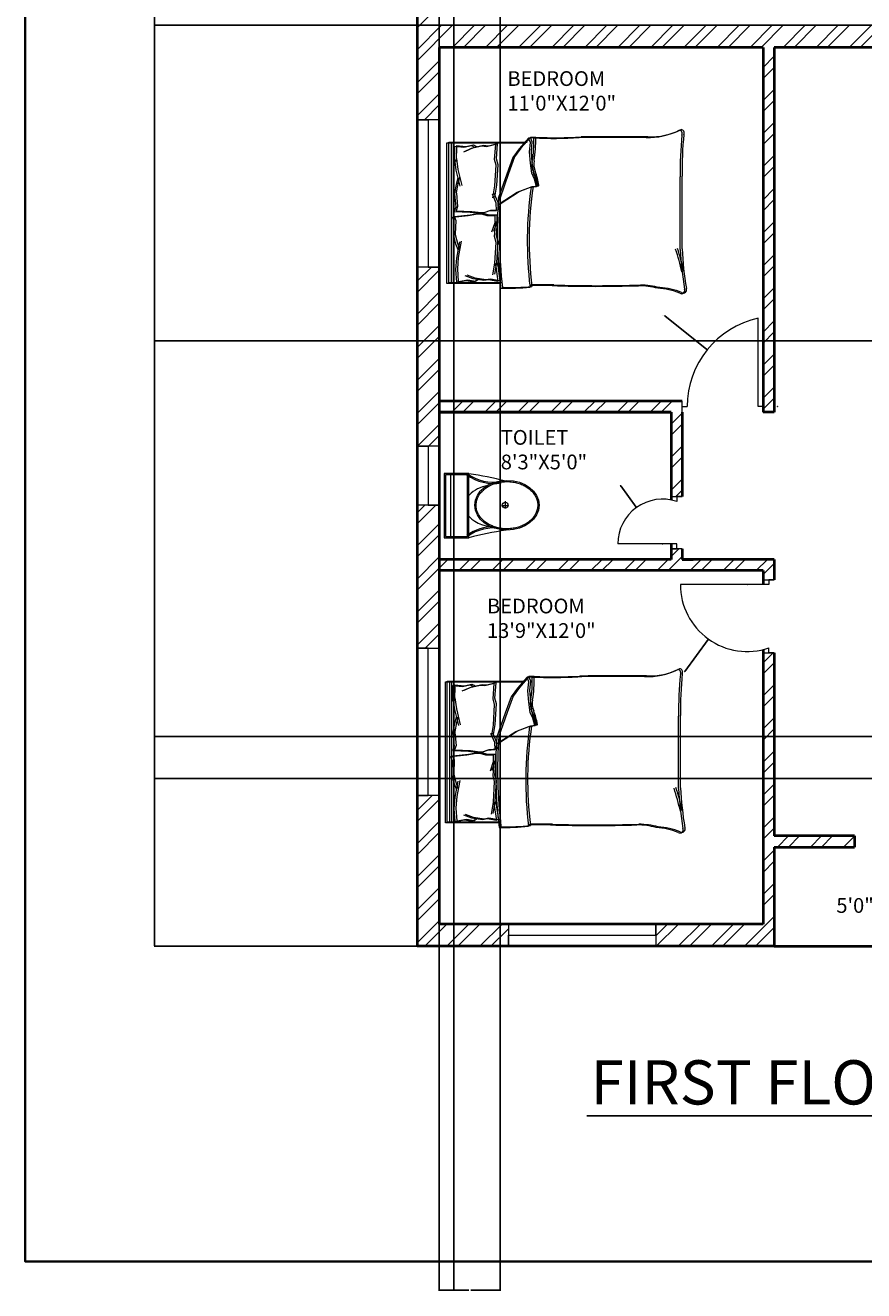
# Model space of a CAD drawing. Units: inches. Extents: x 1355 to 2746, y 1171 to 2751.
# Tile 1 of 24: x 1355 to 1697, y 1171 to 1686. Entities that reach past the tile are written whole.
import ezdxf

# ---------------------------------------------------------------- set-up
doc = ezdxf.new("R2010")
doc.units = ezdxf.units.IN
for name, color, linetype, lineweight in [('A-ANNO-DIMS', 2, 'Continuous', 18), ('A-ANNO-TITL', 7, 'Continuous', 25), ('A-ANNO-TTLB', 7, 'Continuous', 35), ('A-AREA-IDEN', 7, 'Continuous', 18), ('A-DOOR', 3, 'Continuous', 20), ('A-FLOR-FIXT', 9, 'Continuous', 18), ('A-FURN', 8, 'Continuous', 13), ('A-GLAZ', 4, 'Continuous', 18), ('A-WALL', 7, 'Continuous', 40), ('A-WALL-PATT', 252, 'Continuous', 13)]:
    doc.layers.add(name, color=color, linetype=linetype, lineweight=lineweight)
doc.styles.get("Standard").update_dxf_attribs({"font": 'arial.ttf'})
doc.dimstyles.get("Standard").update_dxf_attribs({"dimtxt": 0.18, "dimasz": 0.18, "dimexe": 0.18, "dimexo": 0.0625, "dimgap": 0.09, "dimtad": 0, "dimtih": 1, "dimtoh": 1, "dimdec": 4, "dimzin": 0, "dimdsep": 46, "dimtxsty": 'Standard', "dimcen": 0.09, "dimadec": 0, "dimazin": 0, "dimtfac": 1, "dimtdec": 4, "dimtofl": 0, "dimtmove": 0, "dimatfit": 3, "dimfxl": 1, "dimtolj": 1, "dimtzin": 0, "dimarcsym": 0})

# ---------------------------------------------------------------- blocks, each defined once
blk = doc.blocks.new('A$C31115884')
for p, q in [((258, 466), (258, 523)), ((283, 498), (223, 498)), ((0, 200), (0, 0)), ((520, 200), (0, 200)), ((10, 190), (10, 10)), ((510, 190), (10, 190)), ((510, 10), (510, 190)), ((520, 0), (520, 200)), ((510, 54), (0, 54)), ((10, 10), (510, 10)), ((0, 0), (520, 0))]:
    blk.add_line(p, q)
blk.add_circle((256, 496), 23.6)
for centre, radius, start, end in [((2778, -205), 2807, 165.4549, 171.7133), ((-295, 403), 365, 324.2091, 9.3499), ((-295, 403), 375, 324.2091, 9.3499), ((139, 406), 293, 315.8436, 2.6563), ((806, 403), 365, 170.6501, 215.7909), ((3237, 905), 2807, 188.2867, 194.5451), ((384, 406), 293, 190.2774, 224.1564), ((806, 403), 375, 179.2036, 215.7909)]:
    blk.add_arc(centre, radius, start, end)
blk.add_ellipse((256, 510), major_axis=(0, -261), ratio=0.772727)
blk.add_open_spline([(256, 259), (263, 259), (270, 260), (288, 262), (299, 265), (320, 273), (330, 278), (350, 291), (360, 299), (378, 316), (386, 326), (402, 347), (409, 358), (421, 383), (427, 395), (436, 422), (440, 436), (445, 465), (447, 480), (448, 509), (448, 524), (445, 553), (443, 568), (436, 596), (432, 610), (422, 636), (416, 649), (402, 672), (395, 683), (379, 703), (370, 712), (351, 728), (341, 735), (321, 746), (310, 751), (289, 757), (278, 759), (256, 761), (245, 761), (223, 757), (212, 754), (191, 746), (181, 741), (161, 728), (151, 720), (133, 703), (125, 693), (110, 672), (103, 660), (90, 636), (85, 623), (76, 596), (72, 582), (67, 553), (66, 538), (64, 509), (65, 494), (68, 465), (70, 450), (77, 422), (81, 408), (91, 382), (97, 370), (111, 346), (118, 335), (135, 316), (144, 307), (162, 291), (172, 284), (193, 273), (203, 269), (225, 262), (236, 260), (250, 259), (253, 259), (256, 259)], degree=3, knots=[0, 0, 0, 0, 0.110105, 0.110105, 0.285049, 0.285049, 0.459994, 0.459994, 0.634938, 0.634938, 0.809882, 0.809882, 0.984827, 0.984827, 1.159771, 1.159771, 1.334715, 1.334715, 1.50966, 1.50966, 1.684604, 1.684604, 1.859549, 1.859549, 2.034493, 2.034493, 2.209437, 2.209437, 2.384382, 2.384382, 2.559326, 2.559326, 2.73427, 2.73427, 2.909215, 2.909215, 3.084159, 3.084159, 3.259103, 3.259103, 3.434048, 3.434048, 3.608992, 3.608992, 3.783936, 3.783936, 3.958881, 3.958881, 4.133825, 4.133825, 4.30877, 4.30877, 4.483714, 4.483714, 4.658658, 4.658658, 4.833603, 4.833603, 5.008547, 5.008547, 5.183491, 5.183491, 5.358436, 5.358436, 5.53338, 5.53338, 5.708324, 5.708324, 5.883269, 5.883269, 6.058213, 6.058213, 6.233158, 6.233158, 6.283185, 6.283185, 6.283185, 6.283185])
blk = doc.blocks.new('BED-DOUBLE-PLAN')
for p, q in [((75.16, 62.38), (96.87, 62.38)), ((75.93, 62.66), (97.64, 62.66)), ((86.73, 61.98), (85.52, 61.29)), ((89.85, 61.46), (86.73, 61.98)), ((92.9, 61.88), (89.08, 61.19)), ((93.66, 62.15), (89.85, 61.46)), ((92.87, 61.87), (93.27, 56.74)), ((93.64, 62.15), (94.03, 57.02)), ((95.03, 62.38), (95.03, 5.09)), ((95.8, 62.66), (95.8, 5.36)), ((96.87, 62.38), (96.87, 5.09)), ((97.64, 62.66), (97.64, 5.36)), ((76.95, 55.42), (76.08, 61.53)), ((76.08, 61.53), (79.9, 60.84)), ((77.72, 55.7), (76.85, 61.81)), ((76.85, 61.81), (80.66, 61.11)), ((78.14, 58.9), (77.34, 54.06)), ((78.9, 59.17), (78.1, 54.34)), ((79.9, 60.84), (81.8, 61.19)), ((80.66, 61.11), (82.57, 61.46)), ((81.8, 61.19), (86.14, 60.49)), ((82.57, 61.46), (86.9, 60.77)), ((85.96, 61.71), (84.75, 61.01)), ((89.08, 61.19), (85.96, 61.71)), ((86.14, 60.49), (89.43, 59.28)), ((86.9, 60.77), (90.2, 59.55)), ((93.27, 56.74), (93.24, 56.62)), ((94.01, 56.89), (93.66, 52.31)), ((94.03, 57.02), (94.01, 56.89)), ((77.34, 54.06), (76.82, 45.66)), ((77.34, 54.06), (76.95, 55.42)), ((78.1, 54.34), (77.59, 45.93)), ((78.1, 54.34), (77.72, 55.7)), ((92.9, 52.03), (91.68, 45.45)), ((93.66, 52.31), (92.45, 45.72)), ((93.24, 56.62), (92.9, 52.03)), ((1.87, 48.49), (1.87, 18.98)), ((2.64, 48.76), (2.64, 19.26)), ((92.38, 48.74), (93.24, 46.31)), ((93.14, 49.01), (94.01, 46.59)), ((94.01, 46.59), (94.88, 43.12)), ((76.82, 45.66), (77.49, 43.31)), ((77.49, 43.31), (77, 37.16)), ((77.38, 37.65), (78.68, 41.42)), ((77.59, 45.93), (78.25, 43.58)), ((78.25, 43.58), (77.77, 37.43)), ((78.14, 37.93), (79.45, 41.7)), ((93.24, 46.31), (94.11, 42.85)), ((94.11, 42.46), (93.94, 37.13)), ((94.11, 42.85), (94.11, 42.46)), ((94.88, 42.74), (94.7, 37.41)), ((94.88, 43.12), (94.88, 42.74)), ((77.38, 34.71), (77.38, 37.65)), ((78.14, 34.98), (78.14, 37.93)), ((93.94, 37.13), (94.63, 35.4)), ((94.7, 37.41), (95.4, 35.67)), ((79.83, 32.82), (76.62, 32.62)), ((76.62, 32.62), (76.8, 29.68)), ((80.59, 34.71), (77.38, 34.71)), ((80.6, 33.1), (77.39, 32.9)), ((77.39, 32.9), (77.57, 29.96)), ((81.36, 34.98), (78.14, 34.98)), ((82.03, 33.66), (79.83, 32.82)), ((82.84, 34.01), (80.59, 34.71)), ((82.8, 33.93), (80.6, 33.1)), ((83.61, 34.29), (81.36, 34.98)), ((83.59, 33.75), (82.03, 33.66)), ((84.36, 34.03), (82.8, 33.93)), ((84.4, 34.01), (82.84, 34.01)), ((87.44, 33.3), (83.59, 33.75)), ((85.17, 34.29), (83.61, 34.29)), ((88.21, 33.57), (84.36, 34.03)), ((88.22, 34.71), (84.4, 34.01)), ((88.98, 34.98), (85.17, 34.29)), ((93.89, 33.01), (87.44, 33.3)), ((94.65, 33.28), (88.21, 33.57)), ((94.63, 35.4), (88.22, 34.71)), ((95.4, 35.67), (88.98, 34.98)), ((93.3, 31.24), (93.89, 33.01)), ((93.81, 25.93), (93.3, 31.24)), ((94.07, 31.51), (94.65, 33.28)), ((94.57, 26.2), (94.07, 31.51)), ((76.03, 30.27), (68.25, 25.25)), ((76.8, 30.55), (69.01, 25.52)), ((72.52, 17.82), (76.03, 27.82)), ((73.28, 18.1), (76.8, 28.09)), ((76.8, 29.68), (78.34, 26)), ((78.14, 27.51), (77.34, 22.68)), ((77.57, 29.96), (79.11, 26.28)), ((78.9, 27.78), (78.1, 22.95)), ((93.83, 25.54), (93.81, 25.93)), ((93.95, 22.3), (94.6, 25.82)), ((94.6, 25.82), (94.57, 26.2)), ((62.87, 23.21), (60.45, 22.84)), ((60.45, 22.84), (61.2, 19.86)), ((63.63, 23.48), (61.22, 23.11)), ((61.22, 23.11), (61.96, 20.14)), ((68.25, 25.25), (62.87, 23.21)), ((69.01, 25.52), (63.63, 23.48)), ((77.34, 22.68), (76.82, 14.27)), ((78.1, 22.95), (77.59, 14.54)), ((93.19, 16.3), (91.57, 22.8)), ((93.96, 16.57), (92.34, 23.07)), ((92.47, 19.55), (93.18, 22.03)), ((93.18, 22.03), (93.83, 25.54)), ((93.23, 19.83), (93.95, 22.3)), ((61.2, 19.86), (62.31, 17.45)), ((61.96, 20.14), (63.08, 17.72)), ((62.31, 17.45), (62.87, 13.37)), ((63.08, 17.72), (63.63, 13.64)), ((70.1, 11.14), (72.52, 17.82)), ((70.87, 11.41), (73.28, 18.1)), ((93.82, 11.75), (93.19, 16.3)), ((94.59, 12.02), (93.96, 16.57)), ((62.87, 13.37), (63.24, 8.72)), ((63.63, 13.64), (64, 9)), ((67.51, 7.61), (70.1, 11.14)), ((68.27, 7.88), (70.87, 11.41)), ((76.82, 14.27), (77.49, 11.92)), ((77.49, 11.92), (77, 5.77)), ((77.59, 14.54), (78.25, 12.19)), ((78.25, 12.19), (77.77, 6.04)), ((93.81, 6.47), (93.92, 12.95)), ((93.92, 12.95), (93.82, 11.75)), ((94.57, 6.75), (94.69, 13.22)), ((94.69, 13.22), (94.59, 12.02)), ((63.24, 8.72), (62.87, 5.01)), ((63.61, 3.17), (67.51, 7.61)), ((64, 9), (63.63, 5.28)), ((63.63, 5.28), (64.38, 3.44)), ((64.38, 3.44), (68.27, 7.88)), ((97.64, 5.36), (65.74, 5.36)), ((77, 5.77), (80.77, 6.7)), ((77.77, 6.04), (81.53, 6.97)), ((80.77, 6.7), (82.69, 6.47)), ((81.53, 6.97), (83.46, 6.75)), ((82.69, 6.47), (86.97, 7.43)), ((83.46, 6.75), (87.74, 7.71)), ((86.88, 6.21), (85.62, 6.83)), ((87.64, 6.49), (86.39, 7.1)), ((89.96, 6.93), (86.88, 6.21)), ((86.97, 7.43), (90.18, 8.85)), ((90.72, 7.2), (87.64, 6.49)), ((87.74, 7.71), (90.95, 9.12)), ((93.81, 6.47), (89.96, 6.93)), ((94.57, 6.75), (90.72, 7.2)), ((61.52, 3.07), (63.61, 3.17, 4.64)), ((62.28, 3.35), (64.38, 3.44, 4.64)), ((62.87, 5.01), (63.61, 3.17)), ((96.87, 5.09), (64.97, 5.09))]:
    blk.add_line(p, q)
for centre, radius, start, end in [((1.3, 65.24), 1.31, 56.1736, 203.4781), ((-143.9, 40.86), 145.97, 2.9958, 9.4091), ((2.07, 65.52), 1.31, 56.1736, 203.4781), ((-143.14, 41.13), 145.97, 2.9958, 9.4091), ((12.62, 92.52), 28.25, 247.9751, 266.652), ((13.39, 92.79), 28.25, 247.9751, 266.652), ((19.53, 98.8), 35.53, 256.0648, 268.9113), ((20.29, 99.07), 35.53, 256.0648, 268.9113), ((36.19, -514.68), 578.22, 88.22771, 91.71854), ((36.96, -514.41), 578.22, 88.22771, 91.71854), ((59.5, 267.13), 203.94, 268.4762, 271.0082), ((60.27, 267.4), 203.94, 268.4762, 271.0082), ((-90.53, 45.26), 154.68, 351.7845, 6.9006), ((72.78, -35.55), 99.87, 88.7218, 95.604), ((-89.76, 45.54), 154.68, 351.7845, 6.9006), ((73.55, -35.27), 99.87, 88.7218, 95.604), ((-121.38, 40.94), 197.77, 356.0865, 6.7821), ((-120.62, 41.22), 197.77, 356.0865, 6.7821), ((125.3, 87.2), 127.63, 193.3832, 197.7053), ((126.07, 87.47), 127.63, 193.3832, 197.7053), ((60.38, 22.63), 0.221, 70.2464, 181.1377), ((95.1, 29.2), 35.55, 190.6617, 199.8806), ((61.15, 22.9), 0.221, 70.2464, 181.1377), ((95.86, 29.47), 35.55, 190.6617, 199.8806), ((-157.62, 17.21), 159.5, 354.4998, 0.6351), ((-156.85, 17.49), 159.5, 354.4998, 0.6351), ((54.83, 14.11), 7.46, 348.6608, 23.7384), ((55.6, 14.38), 7.46, 348.6608, 23.7384), ((104.85, 5.01), 43.38, 169.8763, 182.5657), ((105.62, 5.29), 43.38, 169.8763, 182.5657), ((2.32, 1.32), 1.32, 152.6588, 266.02), ((3.08, 1.59), 1.32, 152.6588, 266.02), ((14.55, -24.75), 27.65, 87.4714, 116.4681), ((15.32, -24.48), 27.65, 87.4714, 116.4681), ((15.56, 5471.89), 5469.02, 270.00217, 270.28689), ((16.33, 5472.16), 5469.02, 270.00217, 270.28689), ((53.34, -151.96), 155.25, 86.9791, 93.8365), ((54.1, -151.69), 155.25, 86.9791, 93.8365)]:
    blk.add_arc(centre, radius, start, end)
blk = doc.blocks.new('WINDOW-PLAN-24')
for p, q in [((0, 24), (9, 24)), ((9, 24), (4.5, 24)), ((4.5, 24), (4.5, 0)), ((4.5, 0), (0, 0)), ((0, 0), (9, 0))]:
    blk.add_line(p, q)
blk = doc.blocks.new('WINDOW-PLAN-60')
for p, q in [((0, 60), (9, 60)), ((9, 60), (4.5, 60)), ((4.5, 60), (4.5, 0)), ((4.5, 0), (0, 0)), ((0, 0), (9, 0))]:
    blk.add_line(p, q)
blk = doc.blocks.new('WINDOW-PLAN-60-2')
for p, q in [((4.5, 60), (0, 60)), ((0, 60), (9, 60)), ((4.5, 0), (4.5, 60)), ((9, 0), (0, 0)), ((0, 0), (4.5, 0))]:
    blk.add_line(p, q)
blk = doc.blocks.new('DOOR-BED-SW')
for p, q in [((31, 2.25), (31, 38.25)), ((0, 0), (0, 4.5)), ((0, 2.25), (2, 2.25)), ((33, 2.25), (31, 2.25))]:
    blk.add_line(p, q)
blk.add_arc((38.85, 2.25), 36.84, 102.2933, 180)
blk = doc.blocks.new('DOOR-WC-SW')
for p, q in [((21.75, 21.26), (26.25, 21.26)), ((26.25, 21.26), (24, 21.26)), ((24, 21.26), (24, 19.26)), ((24, 2), (0, 2)), ((24, 0), (24, 2)), ((26.25, 0), (21.75, 0)), ((21.75, 0), (24, 0))]:
    blk.add_line(p, q)
blk.add_arc((18.21, 2), 18.21, 71.4568, 180)
blk = doc.blocks.new('DOOR-BEDROOM-SW')
for p, q in [((36, 27.78), (0, 27.78)), ((33.75, 29.78), (38.25, 29.78)), ((38.25, 29.78), (36, 29.78)), ((36, 29.78), (36, 27.78)), ((33.75, 0), (38.25, 0)), ((36, 0), (36, 2)), ((38.25, 0), (36, 0))]:
    blk.add_line(p, q)
blk.add_arc((27.23, 27.78), 27.23, 180, 288.7918)
blk = doc.blocks.new('*D96')
at = {"layer": 'A-ANNO-DIMS', "color": 0, "lineweight": -2, "transparency": 16777216}
for p, q in [((1514.65, 2139.3), (1407.53, 2139.3)), ((1407.71, 2139.12), (1407.71, 1725.48)), ((1407.71, 1311.48), (1407.71, 1725.12)), ((1514.65, 1311.3), (1407.53, 1311.3))]:
    blk.add_line(p, q, dxfattribs=at)
at = {"layer": 'A-ANNO-DIMS', "color": 0, "transparency": 16777216}
for points in [[(1407.68, 2139.12), (1407.74, 2139.12), (1407.71, 2139.3)], [(1407.68, 1311.48), (1407.74, 1311.48), (1407.71, 1311.3)]]:
    blk.add_solid(points, dxfattribs=at)
at = {"layer": 'Defpoints', "color": 0, "transparency": 16777216}
for p in [(1407.71, 2139.3), (1514.71, 2139.3), (1514.71, 1311.3)]:
    blk.add_point(p, dxfattribs=at)
at = {"layer": 'A-ANNO-DIMS', "color": 0, "transparency": 16777216, "insert": (1407.71, 1725.3), "char_height": 0.18, "attachment_point": 5}
blk.add_mtext('\\A1;828', dxfattribs=at)
blk = doc.blocks.new('*D106')
at = {"layer": 'A-ANNO-DIMS', "color": 0, "lineweight": -2, "transparency": 16777216}
for p, q in [((2031.09, 1557.85), (1407.53, 1557.85)), ((1407.71, 1557.67), (1407.71, 1434.76)), ((1407.71, 1311.48), (1407.71, 1434.39)), ((2080.33, 1311.3), (1407.53, 1311.3))]:
    blk.add_line(p, q, dxfattribs=at)
at = {"layer": 'A-ANNO-DIMS', "color": 0, "transparency": 16777216}
for points in [[(1407.68, 1557.67), (1407.74, 1557.67), (1407.71, 1557.85)], [(1407.68, 1311.48), (1407.74, 1311.48), (1407.71, 1311.3)]]:
    blk.add_solid(points, dxfattribs=at)
at = {"layer": 'Defpoints', "color": 0, "transparency": 16777216}
for p in [(1407.71, 1557.85), (2031.15, 1557.85), (2080.39, 1311.3)]:
    blk.add_point(p, dxfattribs=at)
at = {"layer": 'A-ANNO-DIMS', "color": 0, "transparency": 16777216, "insert": (1407.71, 1434.57), "char_height": 0.18, "attachment_point": 5}
blk.add_mtext('\\A1;246.54', dxfattribs=at)
blk = doc.blocks.new('*D107')
at = {"layer": 'A-ANNO-DIMS', "color": 0, "lineweight": -2, "transparency": 16777216}
for p, q in [((2089.33, 1686.3), (1407.53, 1686.3)), ((1407.71, 1686.12), (1407.71, 1622.26)), ((1407.71, 1558.03), (1407.71, 1621.89)), ((2031.09, 1557.85), (1407.53, 1557.85))]:
    blk.add_line(p, q, dxfattribs=at)
at = {"layer": 'A-ANNO-DIMS', "color": 0, "transparency": 16777216}
for points in [[(1407.68, 1686.12), (1407.74, 1686.12), (1407.71, 1686.3)], [(1407.68, 1558.03), (1407.74, 1558.03), (1407.71, 1557.85)]]:
    blk.add_solid(points, dxfattribs=at)
at = {"layer": 'Defpoints', "color": 0, "transparency": 16777216}
for p in [(1407.71, 1686.3), (2089.39, 1686.3), (2031.15, 1557.85)]:
    blk.add_point(p, dxfattribs=at)
at = {"layer": 'A-ANNO-DIMS', "color": 0, "transparency": 16777216, "insert": (1407.71, 1622.07), "char_height": 0.18, "attachment_point": 5}
blk.add_mtext('\\A1;128.46', dxfattribs=at)
blk = doc.blocks.new('*D137')
at = {"layer": 'A-ANNO-DIMS', "color": 0, "lineweight": -2, "transparency": 16777216}
for p, q in [((1523.71, 1921.74), (1523.71, 1171.06)), ((1529.67, 1919.49), (1529.67, 1171.06)), ((1523.89, 1171.24), (1526.36, 1171.24)), ((1529.49, 1171.24), (1527.01, 1171.24))]:
    blk.add_line(p, q, dxfattribs=at)
at = {"layer": 'A-ANNO-DIMS', "color": 0, "transparency": 16777216}
for points in [[(1523.89, 1171.27), (1523.89, 1171.21), (1523.71, 1171.24)], [(1529.49, 1171.27), (1529.49, 1171.21), (1529.67, 1171.24)]]:
    blk.add_solid(points, dxfattribs=at)
at = {"layer": 'Defpoints', "color": 0, "transparency": 16777216}
for p in [(1523.71, 1921.8), (1529.67, 1919.55), (1529.67, 1171.24)]:
    blk.add_point(p, dxfattribs=at)
at = {"layer": 'A-ANNO-DIMS', "color": 0, "transparency": 16777216, "insert": (1526.69, 1171.24), "char_height": 0.18, "attachment_point": 5}
blk.add_mtext('\\A1;5.96', dxfattribs=at)
blk = doc.blocks.new('*D140')
at = {"layer": 'A-ANNO-DIMS', "color": 0, "lineweight": -2, "transparency": 16777216}
for p, q in [((1523.71, 1973.05), (1523.71, 1171.06)), ((1548.6, 1963.94), (1548.6, 1171.06)), ((1523.89, 1171.24), (1535.76, 1171.24)), ((1548.42, 1171.24), (1536.55, 1171.24))]:
    blk.add_line(p, q, dxfattribs=at)
at = {"layer": 'A-ANNO-DIMS', "color": 0, "transparency": 16777216}
for points in [[(1523.89, 1171.27), (1523.89, 1171.21), (1523.71, 1171.24)], [(1548.42, 1171.27), (1548.42, 1171.21), (1548.6, 1171.24)]]:
    blk.add_solid(points, dxfattribs=at)
at = {"layer": 'Defpoints', "color": 0, "transparency": 16777216}
for p in [(1523.71, 1973.11), (1548.6, 1964.01), (1548.6, 1171.24)]:
    blk.add_point(p, dxfattribs=at)
at = {"layer": 'A-ANNO-DIMS', "color": 0, "transparency": 16777216, "insert": (1536.15, 1171.24), "char_height": 0.18, "attachment_point": 5}
blk.add_mtext('\\A1;24.89', dxfattribs=at)
blk = doc.blocks.new('*D147')
at = {"layer": 'A-ANNO-DIMS', "color": 0, "lineweight": -2, "transparency": 16777216}
for p, q in [((1913.47, 1396.75), (1407.53, 1396.75)), ((1407.71, 1396.57), (1407.71, 1388.37)), ((1407.71, 1379.8), (1407.71, 1388.01)), ((1913.47, 1379.62), (1407.53, 1379.62))]:
    blk.add_line(p, q, dxfattribs=at)
at = {"layer": 'A-ANNO-DIMS', "color": 0, "transparency": 16777216}
for points in [[(1407.68, 1396.57), (1407.74, 1396.57), (1407.71, 1396.75)], [(1407.68, 1379.8), (1407.74, 1379.8), (1407.71, 1379.62)]]:
    blk.add_solid(points, dxfattribs=at)
at = {"layer": 'Defpoints', "color": 0, "transparency": 16777216}
for p in [(1407.71, 1396.75), (1913.53, 1396.75), (1913.53, 1379.62)]:
    blk.add_point(p, dxfattribs=at)
at = {"layer": 'A-ANNO-DIMS', "color": 0, "transparency": 16777216, "insert": (1407.71, 1388.19), "char_height": 0.18, "attachment_point": 5}
blk.add_mtext('\\A1;17.13', dxfattribs=at)
blk = doc.blocks.new('*D153')
at = {"layer": 'A-ANNO-DIMS', "color": 0, "lineweight": -2, "transparency": 16777216}
for p, q in [((1615.46, 1568.03), (1615.64, 1568.03)), ((1615.64, 1568.03), (1632.72, 1554.28)), ((1661.46, 1531.05), (1661.64, 1531.05)), ((1661.55, 1530.96), (1661.55, 1531.14))]:
    blk.add_line(p, q, dxfattribs=at)
at = {"layer": 'A-ANNO-DIMS', "color": 0, "transparency": 16777216}
blk.add_solid([(1632.74, 1554.3), (1632.7, 1554.26), (1632.86, 1554.17)], dxfattribs=at)
at = {"layer": 'Defpoints', "color": 0, "transparency": 16777216}
for p in [(1632.86, 1554.17), (1661.55, 1531.05)]:
    blk.add_point(p, dxfattribs=at)
at = {"layer": 'A-ANNO-DIMS', "color": 0, "transparency": 16777216, "insert": (1614.72, 1568.03), "char_height": 0.18, "attachment_point": 5}
blk.add_mtext('\\A1;2X R36.845', dxfattribs=at)
blk = doc.blocks.new('*D159')
at = {"layer": 'A-ANNO-DIMS', "color": 0, "lineweight": -2, "transparency": 16777216}
for p, q in [((1649.1, 1458.56), (1649.28, 1458.56)), ((1649.19, 1458.47), (1649.19, 1458.65)), ((1623.82, 1423.14), (1633.23, 1436.28)), ((1623.64, 1423.14), (1623.82, 1423.14))]:
    blk.add_line(p, q, dxfattribs=at)
at = {"layer": 'A-ANNO-DIMS', "color": 0, "transparency": 16777216}
blk.add_solid([(1633.21, 1436.3), (1633.25, 1436.26), (1633.33, 1436.42)], dxfattribs=at)
at = {"layer": 'Defpoints', "color": 0, "transparency": 16777216}
for p in [(1649.19, 1458.56), (1633.33, 1436.42)]:
    blk.add_point(p, dxfattribs=at)
at = {"layer": 'A-ANNO-DIMS', "color": 0, "transparency": 16777216, "insert": (1623.16, 1423.14), "char_height": 0.18, "attachment_point": 5}
blk.add_mtext('\\A1;R27.23', dxfattribs=at)
blk = doc.blocks.new('*D164')
at = {"layer": 'A-ANNO-DIMS', "color": 0, "lineweight": -2, "transparency": 16777216}
for p, q in [((1597.47, 1498.8), (1597.65, 1498.8)), ((1597.65, 1498.8), (1603.93, 1490.08)), ((1614.58, 1475.16), (1614.76, 1475.16)), ((1614.67, 1475.07), (1614.67, 1475.25))]:
    blk.add_line(p, q, dxfattribs=at)
at = {"layer": 'A-ANNO-DIMS', "color": 0, "transparency": 16777216}
blk.add_solid([(1603.95, 1490.1), (1603.9, 1490.07), (1604.03, 1489.94)], dxfattribs=at)
at = {"layer": 'Defpoints', "color": 0, "transparency": 16777216}
for p in [(1604.03, 1489.94), (1614.67, 1475.16)]:
    blk.add_point(p, dxfattribs=at)
at = {"layer": 'A-ANNO-DIMS', "color": 0, "transparency": 16777216, "insert": (1597.01, 1498.8), "char_height": 0.18, "attachment_point": 5}
blk.add_mtext('\\A1;R18.21', dxfattribs=at)

msp = doc.modelspace()

# ---------------------------------------------------------------- hatches: boundary and pattern name
at = {"layer": 'A-WALL-PATT'}
h = msp.add_hatch(dxfattribs=at)
h.set_pattern_fill('ANSI32', color=256)
h.paths.add_polyline_path([(1660.2083, 2139.3018), (1614.5977, 2139.3018), (1614.5977, 2130.3018), (1655.7083, 2130.3018), (1655.7083, 1981.8018), (1660.2083, 1981.8018), (1660.2083, 2090.7225), (1692.5832, 2090.7225), (1692.5832, 2095.2225), (1660.2083, 2095.2225)])
h.paths.add_polyline_path([(1523.7083, 2130.3018), (1554.5977, 2130.3018), (1554.5977, 2134.8018), (1554.5977, 2139.3018), (1514.7083, 2139.3018), (1514.7083, 2071.8385), (1523.7083, 2071.8385)])
h.paths.add_polyline_path([(1940.7083, 2139.3018), (1883.7928, 2139.3018), (1883.7928, 2130.3018), (1931.7083, 2130.3018), (1931.7083, 2098.3333), (1940.7083, 2098.3333)])
h.paths.add_polyline_path([(1799.7083, 2130.3018), (1823.7928, 2130.3018), (1823.7928, 2134.8018), (1823.7928, 2139.3018), (1795.2083, 2139.3018), (1795.2083, 2130.3018), (1795.2083, 2095.2225), (1759.2134, 2095.2225), (1759.2134, 2090.7225), (1795.2083, 2090.7225), (1795.2083, 1981.8018), (1799.7083, 1981.8018), (1799.7083, 1986.3018)])
h.paths.add_polyline_path([(1940.7083, 2038.3333), (1931.7083, 2038.3333), (1931.7083, 1986.3018), (1832.7083, 1986.3018), (1832.7083, 1947.1338), (1837.2083, 1947.1338), (1837.2083, 1981.8018), (1931.7083, 1981.8018), (1931.7083, 1967.1939), (1940.7083, 1967.1939)])
h.paths.add_polyline_path([(1940.7083, 1943.1939), (1931.7083, 1943.1939), (1931.7083, 1921.8018), (1837.2083, 1921.8018), (1837.2083, 1926.0511), (1832.7083, 1926.0511), (1832.7083, 1917.3018), (1931.7083, 1917.3018), (1931.7083, 1908.3321), (1940.7083, 1908.3321)])
h.paths.add_polyline_path([(1940.7083, 1884.3321), (1931.7083, 1884.3321), (1931.7083, 1869.3018), (1899.4583, 1869.3018), (1899.4583, 1864.8018), (1931.7083, 1864.8018), (1931.7083, 1773.3018), (1786.5143, 1773.3018), (1786.5143, 1764.3018), (1844.7083, 1764.3018), (1844.7083, 1748.9343), (1853.7083, 1748.9343), (1853.7083, 1764.3018), (1931.7083, 1764.3018), (1931.7083, 1652.9424), (1940.7083, 1652.9424)])
h.paths.add_polyline_path([(1799.7083, 1864.8018), (1806.0522, 1864.8018), (1806.0522, 1867.0518), (1806.0522, 1869.3018), (1799.7083, 1869.3018), (1799.7083, 1917.3018), (1799.7083, 1921.8018), (1795.2083, 1921.8018), (1795.2083, 1773.3018), (1799.7083, 1773.3018)])
h.paths.add_polyline_path([(1872.8988, 1867.0518), (1872.8988, 1869.3018), (1867.2083, 1869.3018), (1867.2083, 1917.3018), (1862.7083, 1917.3018), (1862.7083, 1869.3018), (1836.9546, 1869.3018), (1836.9546, 1864.8018), (1862.7083, 1864.8018), (1872.8988, 1864.8018)])
h.paths.add_polyline_path([(1749.2197, 1773.3018), (1655.7083, 1773.3018), (1523.7083, 1773.3018), (1523.7083, 1828.4963), (1514.7083, 1828.4963), (1514.7083, 1753.9033), (1519.2083, 1753.9033), (1523.7083, 1753.9033), (1523.7083, 1764.3018), (1655.7083, 1764.3018), (1749.2197, 1764.3018), (1749.2197, 1768.8018)])
h.paths.add_polyline_path([(1660.2083, 1921.8018), (1655.7083, 1921.8018), (1655.7083, 1917.3018), (1655.7083, 1773.3018), (1660.2083, 1773.3018)])
h.paths.add_polyline_path([(1523.7083, 2011.8385), (1514.7083, 2011.8385), (1514.7083, 1973.114), (1519.2083, 1973.114), (1523.7083, 1973.114), (1523.7083, 1976.8227), (1523.7083, 1981.8018), (1618.2083, 1981.8018), (1618.2083, 1921.8018), (1553.707, 1921.8018), (1553.707, 1917.3018), (1622.7083, 1917.3018), (1622.7083, 1919.5518), (1622.7083, 1921.8018), (1622.7083, 1986.3018), (1523.7083, 1986.3018)])
h.paths.add_polyline_path([(1529.6686, 1919.5518), (1529.6686, 1921.8018), (1523.7083, 1921.8018), (1523.7083, 1949.114), (1514.7083, 1949.114), (1514.7083, 1888.4963), (1523.7083, 1888.4963), (1523.7083, 1917.3018), (1529.6686, 1917.3018)])
h.paths.add_polyline_path([(1538.9419, 1775.643), (1585.5504, 1775.643), (1585.5504, 1798.0318), (1538.9419, 1798.0318)], flags=25)
h.paths.add_polyline_path([(1696.7097, 1497.3356), (1769.5651, 1497.3356), (1769.5651, 1523.4559), (1696.7097, 1523.4559)], flags=9)
h.paths.add_polyline_path([(1629.1643, 1230.5133), (1877.0879, 1230.5133), (1877.0879, 1267.606), (1629.1643, 1267.606)], flags=9)
h.paths.add_polyline_path([(2533.4462, 2215.4033), (2579.9292, 2215.4033), (2579.9292, 2231.889), (2533.4462, 2231.889)], flags=9)
h.paths.add_polyline_path([(2540.822, 2515.6945), (2594.2245, 2515.6945), (2594.2245, 2545.5463), (2540.822, 2545.5463)], flags=9)
h.paths.add_polyline_path([(2535.9857, 2588.2819), (2582.4687, 2588.2819), (2582.4687, 2604.7675), (2535.9857, 2604.7675)], flags=9)
h.paths.add_polyline_path([(2537.1627, 2617.1172), (2649.1245, 2617.1172), (2649.1245, 2633.6029), (2537.1627, 2633.6029)], flags=9)
h.paths.add_polyline_path([(2218.0051, 2168.228), (2363.9573, 2168.228), (2363.9573, 2205.3208), (2218.0051, 2205.3208)], flags=9)
h.paths.add_polyline_path([(1650.2156, 2165.3631), (1800.3547, 2165.3631), (1800.3547, 2202.4559), (1650.2156, 2202.4559)], flags=9)
h.paths.add_polyline_path([(2553.9592, 1610.7663), (2588.4203, 1610.7663), (2588.4203, 1660.2233), (2553.9592, 1660.2233)], flags=9)
h.paths.add_polyline_path([(1549.0868, 1648.2033), (1595.6952, 1648.2033), (1595.6952, 1670.5921), (1549.0868, 1670.5921)], flags=9)
h.paths.add_polyline_path([(1546.9525, 1502.0931), (1583.3413, 1502.0931), (1583.3413, 1524.4819), (1546.9525, 1524.4819)], flags=9)
h.paths.add_polyline_path([(1540.7704, 1433.4431), (1587.3788, 1433.4431), (1587.3788, 1455.8319), (1540.7704, 1455.8319)], flags=9)
h.paths.add_polyline_path([(1683.6524, 1321.5269), (1760.6169, 1321.5269), (1760.6169, 1333.8911), (1683.6524, 1333.8911)], flags=9)
h.paths.add_polyline_path([(1832.0485, 1356.0874), (1873.0989, 1356.0874), (1873.0989, 1378.4762), (1832.0485, 1378.4762)], flags=9)
h.paths.add_polyline_path([(1877.9694, 1431.2138), (1926.3827, 1431.2138), (1926.3827, 1453.578), (1877.9694, 1453.578)], flags=9)
h.paths.add_polyline_path([(1847.3106, 1499.8371), (1883.6994, 1499.8371), (1883.6994, 1522.2259), (1847.3106, 1522.2259)], flags=9)
h.paths.add_polyline_path([(1813.7015, 1640.7287), (1860.3099, 1640.7287), (1860.3099, 1663.1175), (1813.7015, 1663.1175)], flags=9)
h.paths.add_polyline_path([(1876.2576, 1710.2471), (1912.9452, 1710.2471), (1912.9452, 1732.6359), (1876.2576, 1732.6359)], flags=25)
h.paths.add_polyline_path([(1695.9163, 1715.3064), (1736.9668, 1715.3064), (1736.9668, 1737.6952), (1695.9163, 1737.6952)], flags=9)
h.paths.add_polyline_path([(1881.8583, 1888.9094), (1930.2717, 1888.9094), (1930.2717, 1911.2737), (1881.8583, 1911.2737)], flags=9)
h.paths.add_polyline_path([(1823.9298, 1798.6431), (1864.9803, 1798.6431), (1864.9803, 1821.0319), (1823.9298, 1821.0319)], flags=25)
h.paths.add_polyline_path([(1845.6062, 1948.1408), (1881.995, 1948.1408), (1881.995, 1970.5296), (1845.6062, 1970.5296)], flags=25)
h.paths.add_polyline_path([(1849.027, 1991.5151), (1895.6355, 1991.5151), (1895.6355, 2013.9039), (1849.027, 2013.9039)], flags=25)
h.paths.add_polyline_path([(1684.9725, 2113.8416), (1764.2658, 2113.8416), (1764.2658, 2126.2058), (1684.9725, 2126.2058)], flags=9)
h.paths.add_polyline_path([(1688.6193, 1913.0676), (1776.2005, 1913.0676), (1776.2005, 1935.4564), (1688.6193, 1935.4564)], flags=9)
h.paths.add_polyline_path([(1571.4689, 1930.9816), (1607.8577, 1930.9816), (1607.8577, 1953.3704), (1571.4689, 1953.3704)], flags=25)
h.paths.add_polyline_path([(1535.3581, 1998.3125), (1581.9665, 1998.3125), (1581.9665, 2020.7014), (1535.3581, 2020.7014)], flags=9)
h = msp.add_hatch(dxfattribs=at)
h.set_pattern_fill('ANSI32', color=256)
h.paths.add_polyline_path([(1749.2197, 1686.3018), (1732.6892, 1686.3018), (1523.7083, 1686.3018), (1523.7083, 1705.9033), (1514.7083, 1705.9033), (1514.7083, 1647.8732), (1519.2083, 1647.8732), (1523.7083, 1647.8732), (1523.7083, 1677.3018), (1655.7083, 1677.3018), (1655.7083, 1528.8018), (1660.2083, 1528.8018), (1660.2083, 1677.3018), (1732.6892, 1677.3018), (1749.2197, 1677.3018)])
h.paths.add_polyline_path([(1931.7083, 1686.3018), (1853.7083, 1686.3018), (1853.7083, 1703.5696), (1844.7083, 1703.5696), (1844.7083, 1686.3018), (1788.0274, 1686.3018), (1788.0274, 1677.3018), (1795.2083, 1677.3018), (1795.2083, 1528.8018), (1799.7083, 1528.8018), (1799.7083, 1677.3018), (1844.7083, 1677.3018), (1931.7083, 1677.3018)])
h.paths.add_polyline_path([(1931.7083, 1533.3018), (1844.7083, 1533.3018), (1832.7083, 1533.3018), (1832.7083, 1531.0518), (1832.7083, 1528.8018), (1832.7083, 1495.7519), (1837.2083, 1495.7519), (1837.2083, 1528.8018), (1931.7083, 1528.8018)])
h.paths.add_polyline_path([(1940.7083, 1592.9424), (1931.7083, 1592.9424), (1931.7083, 1506.7845), (1940.7083, 1506.7845)])
h.paths.add_polyline_path([(1940.7083, 1482.7845), (1936.2083, 1482.7845), (1931.7083, 1482.7845), (1931.7083, 1320.3018), (1880.7083, 1320.3018), (1880.7083, 1311.3018), (1940.7083, 1311.3018)])
h.paths.add_polyline_path([(1931.7083, 1468.8018), (1844.7083, 1468.8018), (1837.2083, 1468.8018), (1837.2083, 1474.34), (1832.7083, 1474.34), (1832.7083, 1468.8018), (1832.7083, 1464.3018), (1844.7083, 1464.3018), (1931.7083, 1464.3018)])
h.paths.add_polyline_path([(1863.8571, 1464.3018), (1859.3571, 1464.3018), (1859.3571, 1404.1662), (1838.1542, 1404.1662), (1838.1542, 1399.8018), (1869.4185, 1399.8018), (1869.4185, 1402.0518), (1869.4185, 1404.3018), (1863.8571, 1404.3018)])
h.paths.add_polyline_path([(1799.7083, 1399.6662), (1805.4082, 1399.6662), (1805.4082, 1401.9162), (1805.4082, 1404.1662), (1799.7083, 1404.1662), (1799.7083, 1464.3018), (1799.7083, 1468.8018), (1795.2083, 1468.8018), (1795.2083, 1356.2098), (1761.2597, 1356.2098), (1761.2597, 1351.7098), (1795.2083, 1351.7098), (1795.2083, 1320.3018), (1795.2083, 1311.3018), (1844.7083, 1311.3018), (1844.7083, 1315.8018), (1844.7083, 1320.3018), (1799.7083, 1320.3018)])
h.paths.add_polyline_path([(1692.9218, 1356.2098), (1660.2083, 1356.2098), (1660.2083, 1430.786), (1657.9583, 1430.786), (1655.7083, 1430.786), (1655.7083, 1320.3018), (1611.934, 1320.3018), (1611.934, 1311.3018), (1660.2083, 1311.3018), (1660.2083, 1351.7098), (1692.9218, 1351.7098)])
h.paths.add_polyline_path([(1523.7083, 1372.653), (1514.7083, 1372.653), (1514.7083, 1311.3018), (1551.934, 1311.3018), (1551.934, 1315.8018), (1551.934, 1320.3018), (1523.7083, 1320.3018)])
h.paths.add_polyline_path([(1523.7083, 1490.9023), (1514.7083, 1490.9023), (1514.7083, 1432.653), (1519.2083, 1432.653), (1523.7083, 1432.653)])
h.paths.add_polyline_path([(1660.2083, 1468.8018), (1622.7083, 1468.8018), (1622.7083, 1473.1566), (1618.2083, 1473.1566), (1618.2083, 1468.8018), (1523.7083, 1468.8018), (1523.7083, 1464.3018), (1655.7083, 1464.3018), (1655.7083, 1460.5634), (1660.2083, 1460.5634)])
h.paths.add_polyline_path([(1523.7083, 1587.8732), (1514.7083, 1587.8732), (1514.7083, 1514.9023), (1519.2083, 1514.9023), (1523.7083, 1514.9023)])
h.paths.add_polyline_path([(1622.7083, 1533.3018), (1523.7083, 1533.3018), (1523.7083, 1528.8018), (1618.2083, 1528.8018), (1618.2083, 1494.4205), (1622.7083, 1494.4205), (1622.7083, 1528.8018)])
h.paths.add_polyline_path([(1696.7097, 1497.3356), (1769.5651, 1497.3356), (1769.5651, 1523.4559), (1696.7097, 1523.4559)], flags=9)
h.paths.add_polyline_path([(1629.1643, 1230.5133), (1877.0879, 1230.5133), (1877.0879, 1267.606), (1629.1643, 1267.606)], flags=9)
h.paths.add_polyline_path([(2533.4462, 2215.4033), (2579.9292, 2215.4033), (2579.9292, 2231.889), (2533.4462, 2231.889)], flags=9)
h.paths.add_polyline_path([(2540.822, 2515.6945), (2594.2245, 2515.6945), (2594.2245, 2545.5463), (2540.822, 2545.5463)], flags=9)
h.paths.add_polyline_path([(2535.9857, 2588.2819), (2582.4687, 2588.2819), (2582.4687, 2604.7675), (2535.9857, 2604.7675)], flags=9)
h.paths.add_polyline_path([(2537.1627, 2617.1172), (2649.1245, 2617.1172), (2649.1245, 2633.6029), (2537.1627, 2633.6029)], flags=9)
h.paths.add_polyline_path([(2218.0051, 2168.228), (2363.9573, 2168.228), (2363.9573, 2205.3208), (2218.0051, 2205.3208)], flags=9)
h.paths.add_polyline_path([(1650.2156, 2165.3631), (1800.3547, 2165.3631), (1800.3547, 2202.4559), (1650.2156, 2202.4559)], flags=9)
h.paths.add_polyline_path([(2553.9592, 1610.7663), (2588.4203, 1610.7663), (2588.4203, 1660.2233), (2553.9592, 1660.2233)], flags=9)
h.paths.add_polyline_path([(1549.0868, 1648.2033), (1595.6952, 1648.2033), (1595.6952, 1670.5921), (1549.0868, 1670.5921)], flags=25)
h.paths.add_polyline_path([(1546.9525, 1502.0931), (1583.3413, 1502.0931), (1583.3413, 1524.4819), (1546.9525, 1524.4819)], flags=25)
h.paths.add_polyline_path([(1540.7704, 1433.4431), (1587.3788, 1433.4431), (1587.3788, 1455.8319), (1540.7704, 1455.8319)], flags=9)
h.paths.add_polyline_path([(1683.6524, 1321.5269), (1760.6169, 1321.5269), (1760.6169, 1333.8911), (1683.6524, 1333.8911)], flags=9)
h.paths.add_polyline_path([(1832.0485, 1356.0874), (1873.0989, 1356.0874), (1873.0989, 1378.4762), (1832.0485, 1378.4762)], flags=9)
h.paths.add_polyline_path([(1877.9694, 1431.2138), (1926.3827, 1431.2138), (1926.3827, 1453.578), (1877.9694, 1453.578)], flags=9)
h.paths.add_polyline_path([(1847.3106, 1499.8371), (1883.6994, 1499.8371), (1883.6994, 1522.2259), (1847.3106, 1522.2259)], flags=25)
h.paths.add_polyline_path([(1813.7015, 1640.7287), (1860.3099, 1640.7287), (1860.3099, 1663.1175), (1813.7015, 1663.1175)], flags=25)
h.paths.add_polyline_path([(1876.2576, 1710.2471), (1912.9452, 1710.2471), (1912.9452, 1732.6359), (1876.2576, 1732.6359)], flags=9)
h.paths.add_polyline_path([(1695.9163, 1715.3064), (1736.9668, 1715.3064), (1736.9668, 1737.6952), (1695.9163, 1737.6952)], flags=9)
h.paths.add_polyline_path([(1881.8583, 1888.9094), (1930.2717, 1888.9094), (1930.2717, 1911.2737), (1881.8583, 1911.2737)], flags=9)
h.paths.add_polyline_path([(1823.9298, 1798.6431), (1864.9803, 1798.6431), (1864.9803, 1821.0319), (1823.9298, 1821.0319)], flags=9)
h.paths.add_polyline_path([(1845.6062, 1948.1408), (1881.995, 1948.1408), (1881.995, 1970.5296), (1845.6062, 1970.5296)], flags=9)
h.paths.add_polyline_path([(1849.027, 1991.5151), (1895.6355, 1991.5151), (1895.6355, 2013.9039), (1849.027, 2013.9039)], flags=9)
h.paths.add_polyline_path([(1684.9725, 2113.8416), (1764.2658, 2113.8416), (1764.2658, 2126.2058), (1684.9725, 2126.2058)], flags=9)
h.paths.add_polyline_path([(1688.6193, 1913.0676), (1776.2005, 1913.0676), (1776.2005, 1935.4564), (1688.6193, 1935.4564)], flags=9)
h.paths.add_polyline_path([(1538.9419, 1775.643), (1585.5504, 1775.643), (1585.5504, 1798.0318), (1538.9419, 1798.0318)], flags=9)
h.paths.add_polyline_path([(1571.4689, 1930.9816), (1607.8577, 1930.9816), (1607.8577, 1953.3704), (1571.4689, 1953.3704)], flags=9)
h.paths.add_polyline_path([(1535.3581, 1998.3125), (1581.9665, 1998.3125), (1581.9665, 2020.7014), (1535.3581, 2020.7014)], flags=9)

# ---------------------------------------------------------------- linework, layer by layer
at = {"layer": 'A-ANNO-TITL'}
msp.add_line((1583.8987, 1242.2388), (1821.7611, 1242.2388), dxfattribs=at)
at = {"layer": 'A-ANNO-TTLB'}
msp.add_lwpolyline([(1355.0901, 2751.4741), (2746.1804, 2751.4741), (2746.1804, 1182.883), (1355.0901, 1182.883)], close=True, dxfattribs=at)
at = {"layer": 'A-WALL'}
for p, q in [((1514.7083, 2139.3018), (1514.7083, 1311.3018)), ((1655.7083, 1677.3018), (1523.7083, 1677.3018)), ((1523.7083, 1677.3018), (1523.7083, 1320.3018)), ((1655.7083, 1677.3018), (1655.7083, 1528.8018)), ((1660.2083, 1677.3018), (1660.2083, 1528.8018)), ((1732.6892, 1677.3018), (1660.2083, 1677.3018)), ((1622.7083, 1533.3018), (1523.7083, 1533.3018)), ((1523.7083, 1528.8018), (1618.2083, 1528.8018)), ((1618.2083, 1528.8018), (1523.7083, 1528.8018)), ((1618.2083, 1528.8018), (1618.2083, 1493.0182)), ((1622.7083, 1528.8018), (1622.7083, 1494.4205)), ((1660.2083, 1528.8018), (1655.7083, 1528.8018)), ((1618.2083, 1475.1566), (1618.2083, 1468.8018)), ((1618.2083, 1468.8018), (1523.7083, 1468.8018)), ((1622.7083, 1473.1566), (1622.7083, 1468.8018)), ((1660.2083, 1468.8018), (1622.7083, 1468.8018)), ((1622.7083, 1468.8018), (1627.2083, 1468.8018)), ((1660.2083, 1468.8018), (1660.2083, 1460.5634)), ((1655.7083, 1464.3018), (1523.7083, 1464.3018)), ((1655.7083, 1464.3018), (1655.7083, 1458.5634)), ((1655.7083, 1432.127), (1655.7083, 1320.3018)), ((1660.2083, 1430.786), (1660.2083, 1356.2098)), ((1692.9218, 1356.2098), (1660.2083, 1356.2098)), ((1692.9218, 1356.2098), (1692.9218, 1351.7098)), ((1660.2083, 1351.7098), (1692.9218, 1351.7098)), ((1660.2083, 1351.7098), (1660.2083, 1311.3018)), ((1660.2083, 1351.7098), (1660.2083, 1320.3018)), ((1655.7083, 1320.3018), (1523.7083, 1320.3018)), ((1660.2083, 1311.3018), (1514.7083, 1311.3018)), ((1660.2083, 1311.3018), (1795.2083, 1311.3018))]:
    msp.add_line(p, q, dxfattribs=at)

# ---------------------------------------------------------------- block references
at = {"layer": 'A-DOOR'}
for name, p in [('DOOR-BED-SW', (1622.708, 1528.802)), ('DOOR-WC-SW', (1596.458, 1473.157)), ('DOOR-BEDROOM-SW', (1621.958, 1430.786))]:
    msp.add_blockref(name, p, dxfattribs=at)
at = {"layer": 'A-FLOR-FIXT', "xscale": 0.0501345278177945, "yscale": 0.0501345278177945, "zscale": 0.0501345278177945, "rotation": 270}
msp.add_blockref('A$C31115884', (1525.7382, 1503.7408), dxfattribs=at)
at = {"layer": 'A-FURN', "rotation": 180}
for p in [(1624.5075, 1643.8258), (1623.8786, 1424.2739)]:
    msp.add_blockref('BED-DOUBLE-PLAN', p, dxfattribs=at)
at = {"layer": 'A-GLAZ', "extrusion": (0, 0, -1), "zscale": -1}
for name, p in [('WINDOW-PLAN-60', (-1523.708, 1587.873)), ('WINDOW-PLAN-24', (-1523.708, 1490.902))]:
    msp.add_blockref(name, p, dxfattribs=at)
at = {"layer": 'A-GLAZ'}
msp.add_blockref('WINDOW-PLAN-60-2', (1514.708, 1372.6525), dxfattribs=at)
at = {"layer": 'A-GLAZ', "extrusion": (0, 0, -1), "zscale": -1, "rotation": 270}
msp.add_blockref('WINDOW-PLAN-60', (-1611.934, 1320.302), dxfattribs=at)

# ---------------------------------------------------------------- texts
at = {"layer": 'A-ANNO-TITL', "insert": (1585.3462, 1264.8825), "char_height": 18, "attachment_point": 1}
msp.add_mtext_dynamic_manual_height_columns('FIRST FLOOR PLAN ', width=423.704908, gutter_width=12.5, heights=[0], dxfattribs=at)
at = {"layer": 'A-AREA-IDEN', "char_height": 6, "attachment_point": 1}
for s, width, insert in [('BEDROOM\\P11\'0"X12\'0"', 112.379849, (1551.4994, 1667.6105)), ('TOILET\\P8\'3"X5\'0"', 69.416113, (1548.7922, 1521.5003)), ('BEDROOM\\P13\'9"X12\'0"', 92.20135, (1543.1831, 1452.8504)), ('5\'0" WIDE SIT-OUT', 135.198856, (1685.5003, 1330.9095))]:
    msp.add_mtext_dynamic_manual_height_columns(s, width=width, gutter_width=12.5, heights=[0], dxfattribs=dict(at, insert=insert))

# ---------------------------------------------------------------- dimensions: what is measured, and where the dimension line sits
at = {"layer": 'A-ANNO-DIMS'}
for base, p1, p2, override, picture, middle in [((1407.7083, 2139.3018), (1514.7083, 1311.3018), (1514.7083, 2139.3018), {"dimdec": 0, "dimlfac": 1, "dimrnd": 0, "dimzin": 0, "dimdsep": 46, "dimlunit": 2}, '*D96', (1407.7083, 1725.3018)), ((1407.7083, 1686.3018), (2031.1535, 1557.845), (2089.3909, 1686.3018), {"dimdec": 2, "dimlfac": 1, "dimrnd": 0, "dimzin": 0, "dimdsep": 46, "dimlunit": 2}, '*D107', (1407.7083, 1622.0734)), ((1407.7083, 1557.845), (2080.3909, 1311.3018), (2031.1535, 1557.845), {"dimdec": 2, "dimlfac": 1, "dimrnd": 0, "dimzin": 0, "dimdsep": 46, "dimlunit": 2}, '*D106', (1407.7083, 1434.5734)), ((1407.7083, 1396.7528), (1913.531, 1379.6228), (1913.531, 1396.7528), {"dimdec": 2, "dimlfac": 1, "dimrnd": 0, "dimzin": 0, "dimdsep": 46, "dimlunit": 2}, '*D147', (1407.7083, 1388.1878))]:
    dim = msp.add_linear_dim(base=base, p1=p1, p2=p2, angle=90, dimstyle='Standard', override=override, dxfattribs=at)
    dim.commit()
    dim.dimension.update_dxf_attribs({"geometry": picture, "text_midpoint": middle})
for base, p1, p2, picture, middle in [((1548.5973, 1171.2388), (1523.7077, 1973.1139), (1548.5973, 1964.0069), '*D140', (1536.1525, 1171.2388)), ((1529.6686, 1171.2388), (1523.7083, 1921.8018), (1529.6686, 1919.5518), '*D137', (1526.6885, 1171.2388))]:
    dim = msp.add_linear_dim(base=base, p1=p1, p2=p2, dimstyle='Standard', override={"dimdec": 2, "dimlfac": 1, "dimrnd": 0, "dimzin": 0, "dimdsep": 46, "dimlunit": 2}, dxfattribs=at)
    dim.commit()
    dim.dimension.update_dxf_attribs({"geometry": picture, "text_midpoint": middle})
dim = msp.add_radius_dim(center=(1661.5531, 1531.0518), mpoint=(1632.8602, 1554.1658), text='2X <>', dimstyle='Standard', override={"dimdec": 3, "dimlfac": 1, "dimrnd": 0, "dimzin": 0, "dimdsep": 46, "dimlunit": 2}, dxfattribs=at)
dim.commit()
dim.dimension.update_dxf_attribs({"geometry": '*D153', "text_midpoint": (1614.7191, 1568.0342), "dimtype": 164})
for center, mpoint, picture, middle in [((1614.6674, 1475.1566), (1604.0316, 1489.9368), '*D164', (1597.0076, 1498.8048)), ((1649.1871, 1458.5634), (1633.3349, 1436.4248), '*D159', (1623.1637, 1423.1417))]:
    dim = msp.add_radius_dim(center=center, mpoint=mpoint, dimstyle='Standard', override={"dimdec": 2, "dimlfac": 1, "dimrnd": 0, "dimzin": 0, "dimdsep": 46, "dimlunit": 2}, dxfattribs=at)
    dim.commit()
    dim.dimension.update_dxf_attribs({"geometry": picture, "text_midpoint": middle, "dimtype": 164})

doc.saveas('drawing.dxf')
